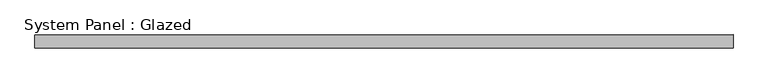
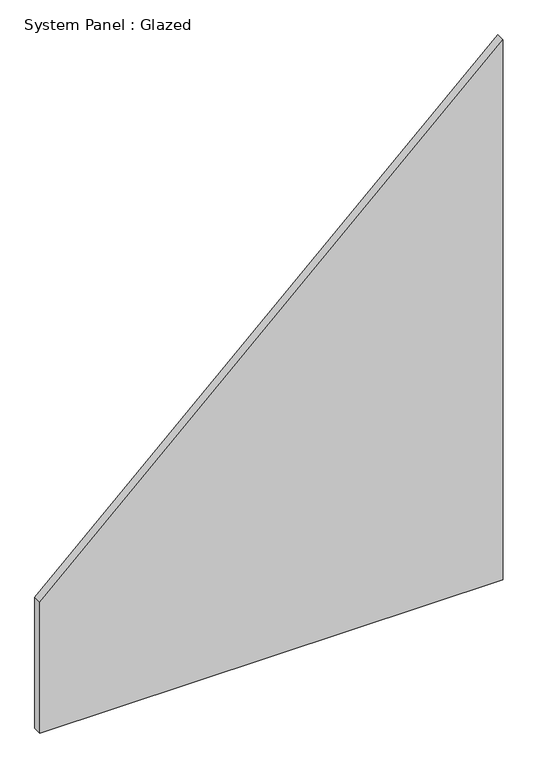
"""IFC4 building model written with IfcOpenShell, lengths in millimetres: plate geometry, System Panel : Glazed."""

from ifc_helpers import new_model, si_unit, frame, origin, place, context, project, spatial, polyline, outline, extrude, source, transform, mapped, element, save


def system_panel_glazed_16cbe3df(model_context):
    return source(origin(), model_context, "Body", "SweptSolid", [
        extrude(outline(polyline([(0.0, -675.1281447), (0.0, 675.1281447), (1662.3468822, 675.1281447), (403.2125222, -675.1281447), (0.0, -675.1281447)])), frame((0.0, 19.05, 0.0), z_axis=(0.0, 1.0, 0.0), x_axis=(0.0, 0.0, 1.0)), (0.0, 0.0, 1.0), 25.4),
    ])


if __name__ == "__main__":
    model = new_model("IFC4")
    model_context = context("Model", 3, world=origin())
    ifc_project = project(units=[si_unit("LENGTHUNIT", "METRE", prefix="MILLI")], contexts=[model_context])
    site = spatial("IfcSite", under=ifc_project)
    building = spatial("IfcBuilding", under=site)
    placement = place(None, origin())
    system_panel_glazed_shape = system_panel_glazed_16cbe3df(model_context)
    element("IfcPlate", 1, ObjectType="System Panel : Glazed", at=placement, inside=building, context=model_context, shape_type="MappedRepresentation", body=[
        mapped(system_panel_glazed_shape, transform((0.0, 0.0, 0.0), x_axis=(1.0, 0.0, 0.0), y_axis=(0.0, 1.0, 0.0), z_axis=(0.0, 0.0, 1.0))),
    ])
    save(model, "model.ifc")

# Revit data of these elements
# Type "System Panel : Glazed"
#   Construction Type Id = "GSP4R"
#   Analytic Construction = "1/8 in Pilkington single glazing"
#   Visual Light Transmittance = 0.9
#   Solar Heat Gain Coefficient = 0.86
#   Heat Transfer Coefficient (U) = 1.18115 BTU/(h·ft²·°F)
#   Define Thermal Properties by = 1
# Element 1 (IfcPlate, "System Panel : Glazed")
#   Materials on its faces: "Glass"
# Materials
#   "Glass": class "Glass", colour RGB 0 128 192, transparency 0.75, Description = "Soda Lime Glass", Cost = 0
